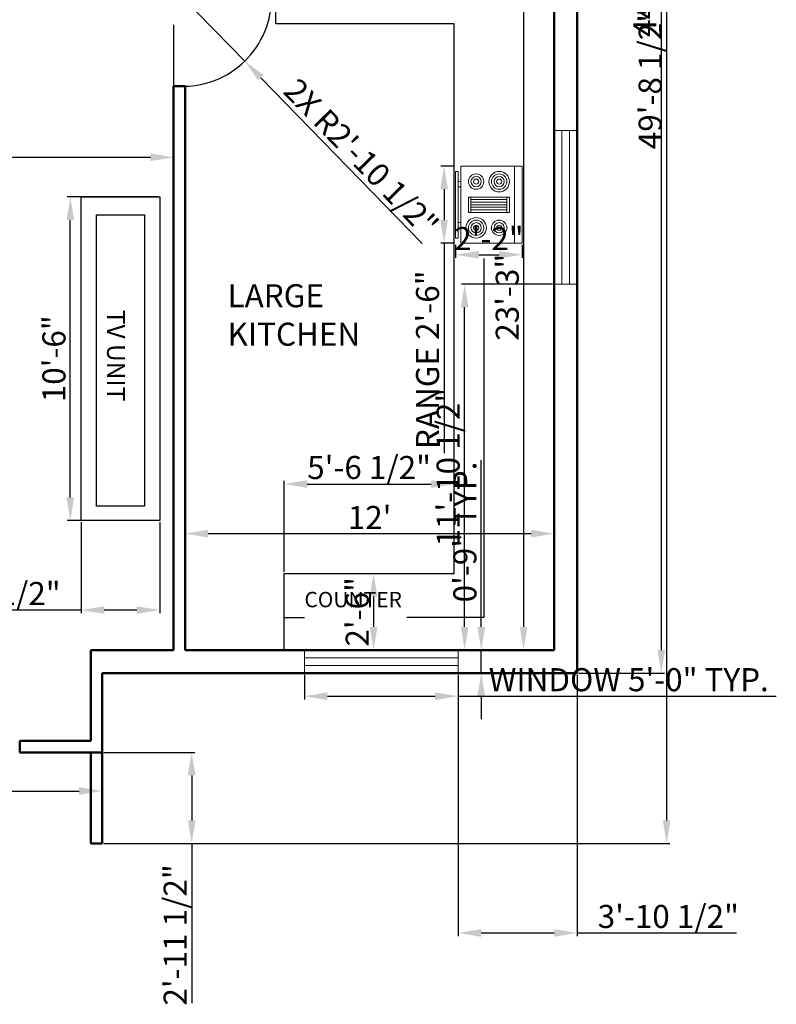
# Model space of a CAD drawing. Units: inches. Extents: x 145135 to 145817, y 90589 to 91373.
# Tile 2 of 4: x 145519 to 145814, y 90589 to 90973. Entities that reach past the tile are written whole.
import ezdxf

# ---------------------------------------------------------------- set-up
doc = ezdxf.new("R2010")
doc.units = ezdxf.units.IN
for name, color, linetype, lineweight in [('A-ANNO-DIMS', 2, 'Continuous', 18), ('A-ANNO-TEXT', 7, 'Continuous', 18), ('A-AREA-IDEN', 7, 'Continuous', 25), ('A-DOOR', 3, 'Continuous', 25), ('A-EQPM', 9, 'Continuous', 18), ('A-FLOR-CASE', 8, 'Continuous', 25), ('A-GLAZ', 4, 'Continuous', 18), ('A-WALL', 7, 'Continuous', 50)]:
    doc.layers.add(name, color=color, linetype=linetype, lineweight=lineweight)
doc.styles.get("Standard").update_dxf_attribs({"font": 'arial.ttf'})
doc.dimstyles.new('ISO-25', dxfattribs={"dimtxt": 9, "dimasz": 9, "dimexe": 1.25, "dimexo": 0.625, "dimtad": 1, "dimdec": 1, "dimrnd": 9, "dimlunit": 3, "dimtxsty": 'Standard', "dimcen": 2.5, "dimadec": 0, "dimazin": 0, "dimtfac": 1, "dimtdec": 1, "dimtmove": 0, "dimatfit": 3, "dimfxl": 1, "dimarcsym": 0})

# ---------------------------------------------------------------- blocks, each defined once
blk = doc.blocks.new('*D16')
at = {"layer": 'A-ANNO-DIMS', "color": 0, "lineweight": -2, "transparency": 16777216}
for p, q in [((145726.81, 91002.52), (145714.28, 91002.52)), ((145715.53, 90993.52), (145715.53, 90736.31)), ((145726.81, 90727.31), (145714.28, 90727.31))]:
    blk.add_line(p, q, dxfattribs=at)
at = {"layer": 'A-ANNO-DIMS', "color": 0, "transparency": 16777216}
for points in [[(145714.03, 90993.52), (145717.03, 90993.52), (145715.53, 91002.52)], [(145714.03, 90736.31), (145717.03, 90736.31), (145715.53, 90727.31)]]:
    blk.add_solid(points, dxfattribs=at)
at = {"layer": 'Defpoints', "color": 0, "transparency": 16777216}
for p in [(145727.43, 91002.52), (145715.53, 90727.31), (145727.43, 90727.31)]:
    blk.add_point(p, dxfattribs=at)
at = {"layer": 'A-ANNO-DIMS', "color": 0, "transparency": 16777216, "insert": (145710.31, 90864.92), "char_height": 9, "attachment_point": 5, "rotation": 90}
blk.add_mtext('23\'-3"', dxfattribs=at)
blk = doc.blocks.new('*D17')
at = {"layer": 'A-ANNO-DIMS', "color": 0, "lineweight": -2, "transparency": 16777216}
for p, q in [((145583.43, 90727.94), (145583.43, 90773.97)), ((145727.43, 90727.94), (145727.43, 90773.97)), ((145592.43, 90772.72), (145718.43, 90772.72))]:
    blk.add_line(p, q, dxfattribs=at)
at = {"layer": 'A-ANNO-DIMS', "color": 0, "transparency": 16777216}
for points in [[(145592.43, 90774.22), (145592.43, 90771.22), (145583.43, 90772.72)], [(145718.43, 90774.22), (145718.43, 90771.22), (145727.43, 90772.72)]]:
    blk.add_solid(points, dxfattribs=at)
at = {"layer": 'Defpoints', "color": 0, "transparency": 16777216}
for p in [(145727.43, 90772.72), (145583.43, 90727.31), (145727.43, 90727.31)]:
    blk.add_point(p, dxfattribs=at)
at = {"layer": 'A-ANNO-DIMS', "color": 0, "transparency": 16777216, "insert": (145655.43, 90777.86), "char_height": 9, "attachment_point": 5}
blk.add_mtext("12'", dxfattribs=at)
blk = doc.blocks.new('*D18')
at = {"layer": 'A-ANNO-DIMS', "color": 0, "lineweight": -2, "transparency": 16777216}
for p, q in [((145350.93, 90971.19), (145350.93, 90918.23)), ((145578.93, 90971.19), (145578.93, 90918.23)), ((145359.93, 90919.48), (145569.93, 90919.48))]:
    blk.add_line(p, q, dxfattribs=at)
at = {"layer": 'A-ANNO-DIMS', "color": 0, "transparency": 16777216}
for points in [[(145359.93, 90920.98), (145359.93, 90917.98), (145350.93, 90919.48)], [(145569.93, 90920.98), (145569.93, 90917.98), (145578.93, 90919.48)]]:
    blk.add_solid(points, dxfattribs=at)
at = {"layer": 'Defpoints', "color": 0, "transparency": 16777216}
for p in [(145350.93, 90971.81), (145578.93, 90971.81), (145578.93, 90919.48)]:
    blk.add_point(p, dxfattribs=at)
at = {"layer": 'A-ANNO-DIMS', "color": 0, "transparency": 16777216, "insert": (145464.93, 90924.7), "char_height": 9, "attachment_point": 5}
blk.add_mtext('18\'-9"', dxfattribs=at)
blk = doc.blocks.new('*D27')
at = {"layer": 'A-ANNO-DIMS', "color": 0, "lineweight": -2, "transparency": 16777216}
for p, q in [((145737.06, 91248.52), (145770.52, 91248.52)), ((145769.27, 91239.52), (145769.27, 90727.31)), ((145737.06, 90718.31), (145770.52, 90718.31))]:
    blk.add_line(p, q, dxfattribs=at)
at = {"layer": 'A-ANNO-DIMS', "color": 0, "transparency": 16777216}
for points in [[(145767.77, 91239.52), (145770.77, 91239.52), (145769.27, 91248.52)], [(145767.77, 90727.31), (145770.77, 90727.31), (145769.27, 90718.31)]]:
    blk.add_solid(points, dxfattribs=at)
at = {"layer": 'Defpoints', "color": 0, "transparency": 16777216}
for p in [(145736.43, 91248.52), (145736.43, 90718.31), (145769.27, 90718.31)]:
    blk.add_point(p, dxfattribs=at)
at = {"layer": 'A-ANNO-DIMS', "color": 0, "transparency": 16777216, "insert": (145764.05, 90983.42), "char_height": 9, "attachment_point": 5, "rotation": 90}
blk.add_mtext('44\'-3"', dxfattribs=at)
blk = doc.blocks.new('*D28')
at = {"layer": 'A-ANNO-DIMS', "color": 0, "lineweight": -2, "transparency": 16777216}
for p, q in [((145383.17, 90686.79), (145383.17, 90671.09)), ((145551.11, 90686.79), (145551.11, 90671.09)), ((145392.17, 90672.34), (145542.11, 90672.34))]:
    blk.add_line(p, q, dxfattribs=at)
at = {"layer": 'A-ANNO-DIMS', "color": 0, "transparency": 16777216}
for points in [[(145392.17, 90673.84), (145392.17, 90670.84), (145383.17, 90672.34)], [(145542.11, 90673.84), (145542.11, 90670.84), (145551.11, 90672.34)]]:
    blk.add_solid(points, dxfattribs=at)
at = {"layer": 'Defpoints', "color": 0, "transparency": 16777216}
for p in [(145383.17, 90687.41), (145551.11, 90687.41), (145551.11, 90672.34)]:
    blk.add_point(p, dxfattribs=at)
at = {"layer": 'A-ANNO-DIMS', "color": 0, "transparency": 16777216, "insert": (145467.14, 90677.57), "char_height": 9, "attachment_point": 5}
blk.add_mtext('14\'-3"', dxfattribs=at)
blk = doc.blocks.new('Range-Oven - 30 in top')
for p, q in [((0, -3), (30, -3)), ((12, -6), (18, -6)), ((13, -20), (13, -6)), ((14, -6), (14, -20)), ((15, -20), (15, -6)), ((16, -6), (16, -20)), ((17, -20), (17, -6)), ((18, -20), (12, -20)), ((6, -24), (6, -25)), ((8, -25), (8, -24)), ((22, -25), (22, -24)), ((24, -24), (24, -25))]:
    blk.add_line(p, q)
for points in [[(0, -24), (0, 0), (30, 0), (30, -24)], [(12, -21), (12, -5), (18, -5), (18, -21)], [(2, -26), (2, -25), (28, -25), (28, -26)]]:
    blk.add_lwpolyline(points, close=True)
for centre, radius in [((6, -9), 4), ((6, -9), 3), ((6, -9), 2), ((24, -9), 3), ((24, -9), 2), ((6, -9), 1), ((24, -9), 1), ((6, -18), 3), ((24, -18), 4), ((24, -18), 3), ((6, -18), 2), ((6, -18), 1), ((24, -18), 2), ((24, -18), 1)]:
    blk.add_circle(centre, radius)
blk = doc.blocks.new('WIN-60IN')
for p, q in [((0, 9), (0, 0)), ((60, 9), (60, 0)), ((60, 6), (0, 6)), ((60, 3), (0, 3))]:
    blk.add_line(p, q)
blk = doc.blocks.new('DOOR-SWING-36IN')
for p, q in [((0, 36.03), (0, 35.03)), ((0, 35.03), (36, 35.03)), ((0, 34.03), (0, 35.03)), ((36, 35.03), (36, 34.03)), ((36, 34.03), (0, 34.03))]:
    blk.add_line(p, q)
blk.add_arc((1.47, 34.53), 34.53, 267.5565, 0.8296)
blk = doc.blocks.new('*D38')
at = {"layer": 'A-ANNO-DIMS', "color": 0, "lineweight": -2, "transparency": 16777216}
for p, q in [((145630, 90717.69), (145630, 90708.06)), ((145690, 90717.69), (145690, 90708.06)), ((145639, 90709.31), (145681, 90709.31)), ((145690, 90709.31), (145814.14, 90709.31))]:
    blk.add_line(p, q, dxfattribs=at)
at = {"layer": 'A-ANNO-DIMS', "color": 0, "transparency": 16777216}
for points in [[(145639, 90710.81), (145639, 90707.81), (145630, 90709.31)], [(145681, 90710.81), (145681, 90707.81), (145690, 90709.31)]]:
    blk.add_solid(points, dxfattribs=at)
at = {"layer": 'Defpoints', "color": 0, "transparency": 16777216}
for p in [(145630, 90718.31), (145690, 90718.31), (145690, 90709.31)]:
    blk.add_point(p, dxfattribs=at)
at = {"layer": 'A-ANNO-DIMS', "color": 0, "transparency": 16777216, "insert": (145756.57, 90714.59), "char_height": 9, "attachment_point": 5}
blk.add_mtext('WINDOW 5\'-0" TYP.', dxfattribs=at)
blk = doc.blocks.new('*D39')
at = {"layer": 'A-ANNO-DIMS', "color": 0, "lineweight": -2, "transparency": 16777216}
for p, q in [((145699, 90736.31), (145699, 90801.42)), ((145690.63, 90727.31), (145700.25, 90727.31)), ((145699, 90718.31), (145699, 90727.31)), ((145690.63, 90718.31), (145700.25, 90718.31)), ((145699, 90709.31), (145699, 90700.31))]:
    blk.add_line(p, q, dxfattribs=at)
at = {"layer": 'A-ANNO-DIMS', "color": 0, "transparency": 16777216}
for points in [[(145697.5, 90736.31), (145700.5, 90736.31), (145699, 90727.31)], [(145697.5, 90709.31), (145700.5, 90709.31), (145699, 90718.31)]]:
    blk.add_solid(points, dxfattribs=at)
at = {"layer": 'Defpoints', "color": 0, "transparency": 16777216}
for p in [(145690, 90727.31), (145699, 90727.31), (145690, 90718.31)]:
    blk.add_point(p, dxfattribs=at)
at = {"layer": 'A-ANNO-DIMS', "color": 0, "transparency": 16777216, "insert": (145693.78, 90773.37), "char_height": 9, "attachment_point": 5, "rotation": 90}
blk.add_mtext('0\'-9" TYP.', dxfattribs=at)
blk = doc.blocks.new('*D52')
at = {"layer": 'A-ANNO-DIMS', "color": 0, "lineweight": -2, "transparency": 16777216}
for p, q in [((145688.38, 90916), (145683.25, 90916)), ((145684.5, 90907), (145684.5, 90895)), ((145688.38, 90886), (145683.25, 90886)), ((145684.5, 90886), (145684.5, 90804.09))]:
    blk.add_line(p, q, dxfattribs=at)
at = {"layer": 'A-ANNO-DIMS', "color": 0, "transparency": 16777216}
for points in [[(145683, 90907), (145686, 90907), (145684.5, 90916)], [(145683, 90895), (145686, 90895), (145684.5, 90886)]]:
    blk.add_solid(points, dxfattribs=at)
at = {"layer": 'Defpoints', "color": 0, "transparency": 16777216}
for p in [(145689, 90916), (145684.5, 90886), (145689, 90886)]:
    blk.add_point(p, dxfattribs=at)
at = {"layer": 'A-ANNO-DIMS', "color": 0, "transparency": 16777216, "insert": (145679.22, 90840.54), "char_height": 9, "attachment_point": 5, "rotation": 90}
blk.add_mtext('RANGE 2\'-6"', dxfattribs=at)
blk = doc.blocks.new('*D53')
at = {"layer": 'A-ANNO-DIMS', "color": 0, "lineweight": -2, "transparency": 16777216}
for p, q in [((145689, 90885.38), (145689, 90880.25)), ((145715, 90885.38), (145715, 90880.25)), ((145698, 90881.5), (145706, 90881.5))]:
    blk.add_line(p, q, dxfattribs=at)
at = {"layer": 'A-ANNO-DIMS', "color": 0, "transparency": 16777216}
for points in [[(145698, 90883), (145698, 90880), (145689, 90881.5)], [(145706, 90883), (145706, 90880), (145715, 90881.5)]]:
    blk.add_solid(points, dxfattribs=at)
at = {"layer": 'Defpoints', "color": 0, "transparency": 16777216}
for p in [(145689, 90886), (145715, 90886), (145715, 90881.5)]:
    blk.add_point(p, dxfattribs=at)
at = {"layer": 'A-ANNO-DIMS', "color": 0, "transparency": 16777216, "insert": (145702, 90886.64), "char_height": 9, "attachment_point": 5}
blk.add_mtext('2\'-2"', dxfattribs=at)
blk = doc.blocks.new('*D60')
at = {"layer": 'A-ANNO-DIMS', "color": 0, "lineweight": -2, "transparency": 16777216}
for p, q in [((145690, 90717.69), (145690, 90615.73)), ((145736.43, 90717.69), (145736.43, 90615.73)), ((145699, 90616.98), (145727.43, 90616.98)), ((145736.43, 90616.98), (145798.57, 90616.98))]:
    blk.add_line(p, q, dxfattribs=at)
at = {"layer": 'A-ANNO-DIMS', "color": 0, "transparency": 16777216}
for points in [[(145699, 90618.48), (145699, 90615.48), (145690, 90616.98)], [(145727.43, 90618.48), (145727.43, 90615.48), (145736.43, 90616.98)]]:
    blk.add_solid(points, dxfattribs=at)
at = {"layer": 'Defpoints', "color": 0, "transparency": 16777216}
for p in [(145690, 90718.31), (145736.43, 90718.31), (145736.43, 90616.98)]:
    blk.add_point(p, dxfattribs=at)
at = {"layer": 'A-ANNO-DIMS', "color": 0, "transparency": 16777216, "insert": (145772, 90622.26), "char_height": 9, "attachment_point": 5}
blk.add_mtext('3\'-10 1/2"', dxfattribs=at)
blk = doc.blocks.new('*D61')
at = {"layer": 'A-ANNO-DIMS', "color": 0, "lineweight": -2, "transparency": 16777216}
for p, q in [((145726.81, 90870), (145691.28, 90870)), ((145692.53, 90736.31), (145692.53, 90861)), ((145726.81, 90727.31), (145691.28, 90727.31))]:
    blk.add_line(p, q, dxfattribs=at)
at = {"layer": 'A-ANNO-DIMS', "color": 0, "transparency": 16777216}
for points in [[(145691.03, 90861), (145694.03, 90861), (145692.53, 90870)], [(145691.03, 90736.31), (145694.03, 90736.31), (145692.53, 90727.31)]]:
    blk.add_solid(points, dxfattribs=at)
at = {"layer": 'Defpoints', "color": 0, "transparency": 16777216}
for p in [(145692.53, 90870), (145727.43, 90870), (145727.43, 90727.31)]:
    blk.add_point(p, dxfattribs=at)
at = {"layer": 'A-ANNO-DIMS', "color": 0, "transparency": 16777216, "insert": (145687.26, 90798.66), "char_height": 9, "attachment_point": 5, "rotation": 90}
blk.add_mtext('11\'-10 1/2"', dxfattribs=at)
blk = doc.blocks.new('*D69')
at = {"layer": 'A-ANNO-DIMS', "color": 0, "lineweight": -2, "transparency": 16777216}
for p, q in [((145551.73, 90687.41), (145587.26, 90687.41)), ((145586.01, 90678.41), (145586.01, 90660.88)), ((145551.73, 90651.88), (145587.26, 90651.88)), ((145586.01, 90651.88), (145586.01, 90589.59))]:
    blk.add_line(p, q, dxfattribs=at)
at = {"layer": 'A-ANNO-DIMS', "color": 0, "transparency": 16777216}
for points in [[(145584.51, 90678.41), (145587.51, 90678.41), (145586.01, 90687.41)], [(145584.51, 90660.88), (145587.51, 90660.88), (145586.01, 90651.88)]]:
    blk.add_solid(points, dxfattribs=at)
at = {"layer": 'Defpoints', "color": 0, "transparency": 16777216}
for p in [(145551.11, 90687.41), (145551.11, 90651.88), (145586.01, 90651.88)]:
    blk.add_point(p, dxfattribs=at)
at = {"layer": 'A-ANNO-DIMS', "color": 0, "transparency": 16777216, "insert": (145580.73, 90616.23), "char_height": 9, "attachment_point": 5, "rotation": 90}
blk.add_mtext('2\'-11 1/2"', dxfattribs=at)
blk = doc.blocks.new('*D70')
at = {"layer": 'A-ANNO-DIMS', "color": 0, "lineweight": -2, "transparency": 16777216}
for p, q in [((145622.72, 90757.16), (145658.24, 90757.16)), ((145656.99, 90748.16), (145656.99, 90736.31)), ((145622.72, 90727.31), (145658.24, 90727.31))]:
    blk.add_line(p, q, dxfattribs=at)
at = {"layer": 'A-ANNO-DIMS', "color": 0, "transparency": 16777216}
for points in [[(145655.49, 90748.16), (145658.49, 90748.16), (145656.99, 90757.16)], [(145655.49, 90736.31), (145658.49, 90736.31), (145656.99, 90727.31)]]:
    blk.add_solid(points, dxfattribs=at)
at = {"layer": 'Defpoints', "color": 0, "transparency": 16777216}
for p in [(145622.09, 90757.16), (145622.09, 90727.31), (145656.99, 90727.31)]:
    blk.add_point(p, dxfattribs=at)
at = {"layer": 'A-ANNO-DIMS', "color": 0, "transparency": 16777216, "insert": (145651.77, 90742.24), "char_height": 9, "attachment_point": 5, "rotation": 90}
blk.add_mtext('2\'-6"', dxfattribs=at)
blk = doc.blocks.new('*D71')
at = {"layer": 'A-ANNO-DIMS', "color": 0, "lineweight": -2, "transparency": 16777216}
for p, q in [((145622.09, 90757.79), (145622.09, 90793.31)), ((145688.4, 90757.79), (145688.4, 90793.31)), ((145631.09, 90792.06), (145679.4, 90792.06))]:
    blk.add_line(p, q, dxfattribs=at)
at = {"layer": 'A-ANNO-DIMS', "color": 0, "transparency": 16777216}
for points in [[(145631.09, 90793.56), (145631.09, 90790.56), (145622.09, 90792.06)], [(145679.4, 90793.56), (145679.4, 90790.56), (145688.4, 90792.06)]]:
    blk.add_solid(points, dxfattribs=at)
at = {"layer": 'Defpoints', "color": 0, "transparency": 16777216}
for p in [(145688.4, 90792.06), (145622.09, 90757.16), (145688.4, 90757.16)]:
    blk.add_point(p, dxfattribs=at)
at = {"layer": 'A-ANNO-DIMS', "color": 0, "transparency": 16777216, "insert": (145655.25, 90797.34), "char_height": 9, "attachment_point": 5}
blk.add_mtext('5\'-6 1/2"', dxfattribs=at)
blk = doc.blocks.new('*D72')
at = {"layer": 'A-ANNO-DIMS', "color": 0, "lineweight": -2, "transparency": 16777216}
for p, q in [((145542.89, 90777.19), (145542.89, 90741.67)), ((145573.55, 90777.19), (145573.55, 90741.67)), ((145542.89, 90742.92), (145487.59, 90742.92)), ((145564.55, 90742.92), (145551.89, 90742.92))]:
    blk.add_line(p, q, dxfattribs=at)
at = {"layer": 'A-ANNO-DIMS', "color": 0, "transparency": 16777216}
for points in [[(145551.89, 90744.42), (145551.89, 90741.42), (145542.89, 90742.92)], [(145564.55, 90744.42), (145564.55, 90741.42), (145573.55, 90742.92)]]:
    blk.add_solid(points, dxfattribs=at)
at = {"layer": 'Defpoints', "color": 0, "transparency": 16777216}
for p in [(145542.89, 90777.82), (145573.55, 90777.82), (145542.89, 90742.92)]:
    blk.add_point(p, dxfattribs=at)
at = {"layer": 'A-ANNO-DIMS', "color": 0, "transparency": 16777216, "insert": (145510.74, 90748.2), "char_height": 9, "attachment_point": 5}
blk.add_mtext('2\'-6 1/2"', dxfattribs=at)
blk = doc.blocks.new('*D73')
at = {"layer": 'A-ANNO-DIMS', "color": 0, "lineweight": -2, "transparency": 16777216}
for p, q in [((145572.92, 90904.03), (145537.4, 90904.03)), ((145538.65, 90786.82), (145538.65, 90895.03)), ((145572.92, 90777.82), (145537.4, 90777.82))]:
    blk.add_line(p, q, dxfattribs=at)
at = {"layer": 'A-ANNO-DIMS', "color": 0, "transparency": 16777216}
for points in [[(145537.15, 90895.03), (145540.15, 90895.03), (145538.65, 90904.03)], [(145537.15, 90786.82), (145540.15, 90786.82), (145538.65, 90777.82)]]:
    blk.add_solid(points, dxfattribs=at)
at = {"layer": 'Defpoints', "color": 0, "transparency": 16777216}
for p in [(145538.65, 90904.03), (145573.55, 90904.03), (145573.55, 90777.82)]:
    blk.add_point(p, dxfattribs=at)
at = {"layer": 'A-ANNO-DIMS', "color": 0, "transparency": 16777216, "insert": (145533.43, 90840.92), "char_height": 9, "attachment_point": 5, "rotation": 90}
blk.add_mtext('10\'-6"', dxfattribs=at)
blk = doc.blocks.new('*D74')
at = {"layer": 'A-ANNO-DIMS', "color": 0, "lineweight": -2, "transparency": 16777216}
for p, q in [((145737.06, 91248.52), (145772.58, 91248.52)), ((145771.33, 91239.52), (145771.33, 90660.88)), ((145551.73, 90651.88), (145772.58, 90651.88))]:
    blk.add_line(p, q, dxfattribs=at)
at = {"layer": 'A-ANNO-DIMS', "color": 0, "transparency": 16777216}
for points in [[(145769.83, 91239.52), (145772.83, 91239.52), (145771.33, 91248.52)], [(145769.83, 90660.88), (145772.83, 90660.88), (145771.33, 90651.88)]]:
    blk.add_solid(points, dxfattribs=at)
at = {"layer": 'Defpoints', "color": 0, "transparency": 16777216}
for p in [(145736.43, 91248.52), (145551.11, 90651.88), (145771.33, 90651.88)]:
    blk.add_point(p, dxfattribs=at)
at = {"layer": 'A-ANNO-DIMS', "color": 0, "transparency": 16777216, "insert": (145766.06, 90950.2), "char_height": 9, "attachment_point": 5, "rotation": 90}
blk.add_mtext('49\'-8 1/2"', dxfattribs=at)
blk = doc.blocks.new('*D78')
at = {"layer": 'A-ANNO-DIMS', "color": 0, "lineweight": -2, "transparency": 16777216}
for p, q in [((145582.66, 90981.74), (145606.73, 90956.98)), ((145675.91, 90885.83), (145613, 90950.53))]:
    blk.add_line(p, q, dxfattribs=at)
at = {"layer": 'A-ANNO-DIMS', "color": 0, "transparency": 16777216}
blk.add_solid([(145614.08, 90951.57), (145611.93, 90949.48), (145606.73, 90956.98)], dxfattribs=at)
at = {"layer": 'Defpoints', "color": 0, "transparency": 16777216}
for p in [(145582.66, 90981.74), (145606.73, 90956.98)]:
    blk.add_point(p, dxfattribs=at)
at = {"layer": 'A-ANNO-DIMS', "color": 0, "transparency": 16777216, "insert": (145651.38, 90918.63), "char_height": 9, "attachment_point": 5, "rotation": 314.1935}
blk.add_mtext('2X R2\'-10 1/2"', dxfattribs=at)

msp = doc.modelspace()

# ---------------------------------------------------------------- linework, layer by layer
at = {"layer": 'A-FLOR-CASE'}
for p, q in [((145618.84, 90971.55), (145618.84, 91002.52)), ((145688.4, 90971.55), (145618.84, 90971.55)), ((145688.4, 90757.16), (145688.4, 90971.55)), ((145700, 90880), (145700, 90740)), ((145622.09, 90727.31), (145622.09, 90757.16)), ((145622.09, 90757.16), (145688.4, 90757.16)), ((145622.09, 90740), (145622.09, 90740)), ((145622.09, 90740), (145630, 90740)), ((145700, 90740), (145670, 90740))]:
    msp.add_line(p, q, dxfattribs=at)
for points in [[(145542.89, 90904.03), (145573.55, 90904.03), (145573.55, 90777.82), (145542.89, 90777.82)], [(145548.84, 90897.07), (145567.58, 90897.07), (145567.58, 90783.43), (145548.84, 90783.43)]]:
    msp.add_lwpolyline(points, close=True, dxfattribs=at)
at = {"layer": 'A-WALL'}
for p, q in [((145736.43, 90718.31), (145736.43, 91248.52)), ((145727.43, 90727.31), (145727.43, 91002.52)), ((145578.93, 90727.31), (145578.93, 90947.24)), ((145578.93, 90947.24), (145583.43, 90947.24)), ((145583.43, 90727.31), (145583.43, 90947.24)), ((145546.61, 90691.91), (145546.61, 90727.31)), ((145546.61, 90727.31), (145578.93, 90727.31)), ((145583.43, 90727.31), (145727.43, 90727.31)), ((145551.11, 90687.41), (145551.11, 90718.31)), ((145551.11, 90718.31), (145727.43, 90718.31)), ((145727.43, 90718.31), (145736.43, 90718.31)), ((145518.95, 90691.91), (145518.95, 90687.41)), ((145518.95, 90691.91), (145546.61, 90691.91)), ((145518.95, 90687.41), (145551.11, 90687.41)), ((145546.61, 90651.88), (145546.61, 90687.41)), ((145551.11, 90651.88), (145551.11, 90687.41)), ((145546.61, 90651.88), (145551.11, 90651.88))]:
    msp.add_line(p, q, dxfattribs=at)

# ---------------------------------------------------------------- block references
at = {"layer": 'A-DOOR'}
msp.add_blockref('DOOR-SWING-36IN', (145581.18, 90947.21), dxfattribs=at)
at = {"layer": 'A-EQPM', "rotation": 270}
msp.add_blockref('Range-Oven - 30 in top', (145715, 90916), dxfattribs=at)
at = {"layer": 'A-GLAZ', "rotation": 89.99999999994564}
msp.add_blockref('WIN-60IN', (145736.43, 90870), dxfattribs=at)
at = {"layer": 'A-GLAZ'}
msp.add_blockref('WIN-60IN', (145630, 90718.31), dxfattribs=at)

# ---------------------------------------------------------------- texts
at = {"layer": 'A-ANNO-TEXT', "insert": (145560, 90860), "char_height": 7, "attachment_point": 1, "rotation": 270}
msp.add_mtext_dynamic_manual_height_columns('TV UNIT', width=520, gutter_width=12.5, heights=[0], dxfattribs=at)
at = {"layer": 'A-ANNO-TEXT', "insert": (145630, 90750), "char_height": 6, "attachment_point": 1}
msp.add_mtext_dynamic_manual_height_columns('COUNTER', width=50, gutter_width=12.5, heights=[0], dxfattribs=at)
at = {"layer": 'A-AREA-IDEN', "insert": (145600, 90870), "char_height": 9, "attachment_point": 1}
msp.add_mtext_dynamic_manual_height_columns('LARGE KITCHEN', width=90, gutter_width=12.5, heights=[0], dxfattribs=at)

# ---------------------------------------------------------------- dimensions: what is measured, and where the dimension line sits
at = {"layer": 'A-ANNO-DIMS'}
for base, p1, p2, angle, override, picture, middle in [((145771.33, 90651.88), (145736.43, 91248.52), (145551.11, 90651.88), 90, {"dimdec": 1, "dimlfac": 1, "dimrnd": 0, "dimzin": 1, "dimdsep": 46, "dimlunit": 4, "dimfrac": 2}, '*D74', (145766.06, 90950.2)), ((145769.27, 90718.31), (145736.43, 91248.52), (145736.43, 90718.31), 90, {"dimclrd": 0, "dimclre": 0, "dimclrt": 0}, '*D27', (145764.05, 90983.42)), ((145715.53, 90727.31), (145727.43, 91002.52), (145727.43, 90727.31), 90, {"dimclrd": 0, "dimclre": 0, "dimclrt": 0}, '*D16', (145710.31, 90864.92)), ((145538.65, 90904.03), (145573.55, 90777.82), (145573.55, 90904.03), 90, {"dimdec": 1, "dimlfac": 1, "dimrnd": 0, "dimzin": 1, "dimdsep": 46, "dimlunit": 4, "dimfrac": 2}, '*D73', (145533.43, 90840.92)), ((145692.53, 90870), (145727.43, 90727.31), (145727.43, 90870), 90, {"dimdec": 1, "dimlfac": 1, "dimrnd": 0, "dimzin": 1, "dimdsep": 46, "dimlunit": 4, "dimfrac": 2}, '*D61', (145687.26, 90798.66)), ((145542.89, 90742.92), (145573.55, 90777.82), (145542.89, 90777.82), 180, {"dimdec": 1, "dimlfac": 1, "dimrnd": 0, "dimzin": 1, "dimdsep": 46, "dimlunit": 4, "dimfrac": 2}, '*D72', (145510.74, 90748.2)), ((145656.9928, 90727.3129), (145622.0928, 90757.1621), (145622.0928, 90727.3129), 270, {"dimdec": 1, "dimlfac": 1, "dimrnd": 0, "dimzin": 1, "dimdsep": 46, "dimlunit": 4, "dimfrac": 2}, '*D70', (145651.7726, 90742.2375)), ((145586.01, 90651.88), (145551.11, 90687.41), (145551.11, 90651.88), 270, {"dimdec": 1, "dimlfac": 1, "dimrnd": 0, "dimzin": 1, "dimdsep": 46, "dimlunit": 4, "dimfrac": 2}, '*D69', (145580.73, 90616.23))]:
    dim = msp.add_linear_dim(base=base, p1=p1, p2=p2, angle=angle, dimstyle='ISO-25', override=override, dxfattribs=at)
    dim.commit()
    dim.dimension.update_dxf_attribs({"geometry": picture, "text_midpoint": middle})
dim = msp.add_radius_dim(center=(145582.66, 90981.74), mpoint=(145606.73, 90956.98), text='2X <>', dimstyle='ISO-25', override={"dimdec": 1, "dimlfac": 1, "dimrnd": 0, "dimzin": 1, "dimdsep": 46, "dimlunit": 4, "dimfrac": 2}, dxfattribs=at)
dim.commit()
dim.dimension.update_dxf_attribs({"geometry": '*D78', "text_midpoint": (145651.38, 90918.63)})
for base, p1, p2, override, picture, middle in [((145578.93, 90919.48), (145350.93, 90971.81), (145578.93, 90971.81), {"dimclrd": 0, "dimclre": 0, "dimclrt": 0}, '*D18', (145464.93, 90924.7)), ((145715, 90881.5), (145689, 90886), (145715, 90886), {"dimdec": 1, "dimlfac": 1, "dimrnd": 0, "dimzin": 1, "dimdsep": 46, "dimlunit": 4, "dimfrac": 2}, '*D53', (145702, 90886.64)), ((145688.4, 90792.06), (145622.09, 90757.16), (145688.4, 90757.16), {"dimdec": 1, "dimlfac": 1, "dimrnd": 0, "dimzin": 1, "dimdsep": 46, "dimlunit": 4, "dimfrac": 2}, '*D71', (145655.25, 90797.34)), ((145727.43, 90772.72), (145583.43, 90727.31), (145727.43, 90727.31), {"dimclrd": 0, "dimclre": 0, "dimclrt": 0}, '*D17', (145655.43, 90777.86)), ((145736.43, 90616.98), (145690, 90718.31), (145736.43, 90718.31), {"dimdec": 1, "dimlfac": 1, "dimrnd": 0, "dimzin": 1, "dimdsep": 46, "dimlunit": 4, "dimfrac": 2}, '*D60', (145772, 90622.26)), ((145551.11, 90672.34), (145383.17, 90687.41), (145551.11, 90687.41), {"dimclrd": 0, "dimclre": 0, "dimclrt": 0}, '*D28', (145467.14, 90677.57))]:
    dim = msp.add_linear_dim(base=base, p1=p1, p2=p2, dimstyle='ISO-25', override=override, dxfattribs=at)
    dim.commit()
    dim.dimension.update_dxf_attribs({"geometry": picture, "text_midpoint": middle})
for base, p1, p2, angle, text, picture, middle in [((145684.5, 90886), (145689, 90916), (145689, 90886), 270, 'RANGE <>', '*D52', (145679.22, 90840.54)), ((145699, 90727.31), (145690, 90718.31), (145690, 90727.31), 90, '<> TYP.', '*D39', (145693.78, 90773.37))]:
    dim = msp.add_linear_dim(base=base, p1=p1, p2=p2, angle=angle, text=text, dimstyle='ISO-25', override={"dimdec": 1, "dimlfac": 1, "dimrnd": 0, "dimzin": 1, "dimdsep": 46, "dimlunit": 4, "dimfrac": 2}, dxfattribs=at)
    dim.commit()
    dim.dimension.update_dxf_attribs({"geometry": picture, "text_midpoint": middle})
dim = msp.add_linear_dim(base=(145690, 90709.31), p1=(145630, 90718.31), p2=(145690, 90718.31), text='WINDOW <> TYP.', dimstyle='ISO-25', override={"dimdec": 1, "dimlfac": 1, "dimrnd": 0, "dimzin": 1, "dimdsep": 46, "dimlunit": 4, "dimfrac": 2}, dxfattribs=at)
dim.commit()
dim.dimension.update_dxf_attribs({"geometry": '*D38', "text_midpoint": (145756.57, 90714.59)})

doc.saveas('drawing.dxf')
